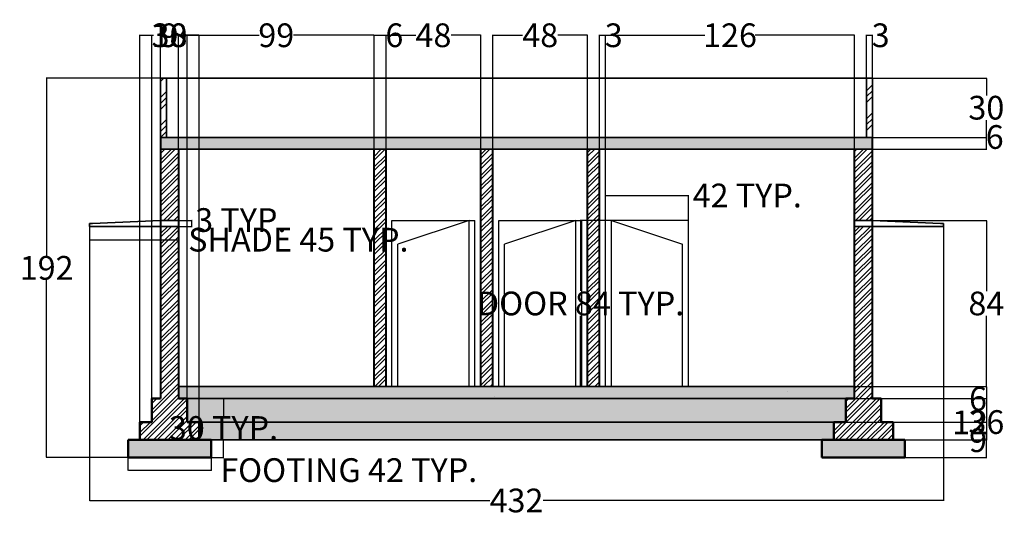
# Model space of a CAD drawing. Units: inches. Extents: x -51 to 1196, y -40 to 252.
# Tile 1 of 2: x -51 to 447, y -40 to 215. Entities that reach past the tile are written whole.
import ezdxf

# ---------------------------------------------------------------- set-up
doc = ezdxf.new("R2010")
doc.units = ezdxf.units.IN
doc.header["$MEASUREMENT"] = 0
for name, color, linetype, lineweight in [('A-ANNO-DIMS', 2, 'Continuous', 18), ('A-DOOR', 4, 'Continuous', 25), ('A-FLOR', 7, 'Continuous', 35), ('A-FLOR-PATT', 8, 'Continuous', 13), ('A-ROOF', 7, 'Continuous', 35), ('A-ROOF-PATT', 8, 'Continuous', 13), ('A-SECT-PATT', 8, 'Continuous', 13), ('A-WALL', 7, 'Continuous', 40), ('S-FNDN', 1, 'Continuous', 50), ('S-FNDN-PATT', 8, 'Continuous', 13)]:
    doc.layers.add(name, color=color, linetype=linetype, lineweight=lineweight)
doc.styles.get("Standard").update_dxf_attribs({"font": 'arial.ttf'})
doc.dimstyles.get("Standard").update_dxf_attribs({"dimtxt": 12, "dimasz": 0.18, "dimexe": 0.18, "dimexo": 0.0625, "dimgap": 0.09, "dimtad": 0, "dimtih": 1, "dimtoh": 1, "dimdec": 0, "dimzin": 0, "dimdsep": 46, "dimlunit": 4, "dimtxsty": 'Standard', "dimcen": 0.09, "dimadec": 0, "dimazin": 0, "dimtfac": 1, "dimtdec": 0, "dimtofl": 0, "dimtmove": 0, "dimatfit": 3, "dimfxl": 1, "dimtolj": 1, "dimtzin": 0, "dimarcsym": 0})

# ---------------------------------------------------------------- blocks, each defined once
blk = doc.blocks.new('DOOR-42X84-SECTION')
for p, q in [((42, 84), (0, 84)), ((0, 0), (0, 84)), ((3, 0), (3, 84)), ((3, 84), (39, 72)), ((42, 0), (42, 84)), ((39, 0), (39, 72))]:
    blk.add_line(p, q)
blk = doc.blocks.new('FOOTING-STEPPED-42')
for p, q in [((12, 30), (12, 18)), ((16.5, 30), (12, 30)), ((30, 30), (25.5, 30)), ((30, 18), (30, 30)), ((12, 18), (6, 18)), ((6, 18), (6, 9)), ((36, 18), (30, 18)), ((36, 9), (36, 18)), ((6, 9), (0, 9)), ((0, 9), (0, 0)), ((6, 9), (36, 9)), ((42, 9), (36, 9)), ((42, 0), (42, 9)), ((0, 0), (42, 0))]:
    blk.add_line(p, q)
blk = doc.blocks.new('SHADE-PROJECTING-36')
for p, q in [((0, 0), (0, 1.5)), ((0, 1.5), (1.5, 1.5)), ((36, 0), (0, 0)), ((1.5, 1.5), (36, 3)), ((45, 3), (36, 3)), ((45, 0), (36, 0))]:
    blk.add_line(p, q)
blk = doc.blocks.new('*D6')
at = {"layer": 'A-ANNO-DIMS', "color": 0, "lineweight": -2, "transparency": 16777216}
for p, q in [((245.36, 113.83), (232.64, 113.83)), ((232.82, 113.65), (232.82, 78.13)), ((232.82, 30.01), (232.82, 65.53)), ((245.36, 29.83), (232.64, 29.83))]:
    blk.add_line(p, q, dxfattribs=at)
at = {"layer": 'A-ANNO-DIMS', "color": 0, "transparency": 16777216}
for points in [[(232.79, 113.65), (232.85, 113.65), (232.82, 113.83)], [(232.79, 30.01), (232.85, 30.01), (232.82, 29.83)]]:
    blk.add_solid(points, dxfattribs=at)
at = {"layer": 'Defpoints', "color": 0, "transparency": 16777216}
for p in [(232.82, 113.83), (245.42, 113.83), (245.42, 29.83)]:
    blk.add_point(p, dxfattribs=at)
at = {"layer": 'A-ANNO-DIMS', "color": 0, "transparency": 16777216, "insert": (232.82, 71.83), "char_height": 12, "attachment_point": 5}
blk.add_mtext('\\A1;DOOR 84 TYP.', dxfattribs=at)
blk = doc.blocks.new('*D7')
at = {"layer": 'A-ANNO-DIMS', "color": 0, "lineweight": -2, "transparency": 16777216}
for p, q in [((245.42, 113.89), (245.42, 126.61)), ((245.6, 126.43), (287.24, 126.43)), ((287.42, 113.89), (287.42, 126.61)), ((287.42, 126.43), (287.6, 126.43))]:
    blk.add_line(p, q, dxfattribs=at)
at = {"layer": 'A-ANNO-DIMS', "color": 0, "transparency": 16777216}
for points in [[(245.6, 126.46), (245.6, 126.4), (245.42, 126.43)], [(287.24, 126.46), (287.24, 126.4), (287.42, 126.43)]]:
    blk.add_solid(points, dxfattribs=at)
at = {"layer": 'Defpoints', "color": 0, "transparency": 16777216}
for p in [(287.42, 126.43), (245.42, 113.83), (287.42, 113.83)]:
    blk.add_point(p, dxfattribs=at)
at = {"layer": 'A-ANNO-DIMS', "color": 0, "transparency": 16777216, "insert": (317.14, 126.43), "char_height": 12, "attachment_point": 5}
blk.add_mtext('\\A1;42 TYP.', dxfattribs=at)
blk = doc.blocks.new('*D8')
at = {"layer": 'A-ANNO-DIMS', "color": 0, "lineweight": -2, "transparency": 16777216}
for p, q in [((3.92, -6.24), (3.92, -12.65)), ((45.92, -6.24), (45.92, -12.65)), ((4.1, -12.47), (45.74, -12.47)), ((45.92, -12.47), (46.1, -12.47))]:
    blk.add_line(p, q, dxfattribs=at)
at = {"layer": 'A-ANNO-DIMS', "color": 0, "transparency": 16777216}
for points in [[(4.1, -12.44), (4.1, -12.5), (3.92, -12.47)], [(45.74, -12.44), (45.74, -12.5), (45.92, -12.47)]]:
    blk.add_solid(points, dxfattribs=at)
at = {"layer": 'Defpoints', "color": 0, "transparency": 16777216}
for p in [(3.92, -6.17), (45.92, -6.17), (45.92, -12.47)]:
    blk.add_point(p, dxfattribs=at)
at = {"layer": 'A-ANNO-DIMS', "color": 0, "transparency": 16777216, "insert": (115.57, -12.47), "char_height": 12, "attachment_point": 5}
blk.add_mtext('\\A1;FOOTING 42 TYP.', dxfattribs=at)
blk = doc.blocks.new('*D9')
at = {"layer": 'A-ANNO-DIMS', "color": 0, "lineweight": -2, "transparency": 16777216}
for p, q in [((45.98, 23.83), (52.4, 23.83)), ((52.22, 23.65), (52.22, 15.05)), ((52.22, -5.99), (52.22, 2.61)), ((45.98, -6.17), (52.4, -6.17))]:
    blk.add_line(p, q, dxfattribs=at)
at = {"layer": 'A-ANNO-DIMS', "color": 0, "transparency": 16777216}
for points in [[(52.19, 23.65), (52.25, 23.65), (52.22, 23.83)], [(52.19, -5.99), (52.25, -5.99), (52.22, -6.17)]]:
    blk.add_solid(points, dxfattribs=at)
at = {"layer": 'Defpoints', "color": 0, "transparency": 16777216}
for p in [(45.92, 23.83), (52.22, 23.83), (45.92, -6.17)]:
    blk.add_point(p, dxfattribs=at)
at = {"layer": 'A-ANNO-DIMS', "color": 0, "transparency": 16777216, "insert": (52.22, 8.83), "char_height": 12, "attachment_point": 5}
blk.add_mtext('\\A1;30 TYP.', dxfattribs=at)
blk = doc.blocks.new('*D10')
at = {"layer": 'A-ANNO-DIMS', "color": 0, "lineweight": -2, "transparency": 16777216}
for p, q in [((-15.58, 110.76), (-15.58, 103.9)), ((29.42, 110.76), (29.42, 103.9)), ((-15.4, 104.08), (29.24, 104.08)), ((29.42, 104.08), (29.6, 104.08))]:
    blk.add_line(p, q, dxfattribs=at)
at = {"layer": 'A-ANNO-DIMS', "color": 0, "transparency": 16777216}
for points in [[(-15.4, 104.11), (-15.4, 104.05), (-15.58, 104.08)], [(29.24, 104.11), (29.24, 104.05), (29.42, 104.08)]]:
    blk.add_solid(points, dxfattribs=at)
at = {"layer": 'Defpoints', "color": 0, "transparency": 16777216}
for p in [(-15.58, 110.83), (29.42, 110.83), (29.42, 104.08)]:
    blk.add_point(p, dxfattribs=at)
at = {"layer": 'A-ANNO-DIMS', "color": 0, "transparency": 16777216, "insert": (90.08, 104.08), "char_height": 12, "attachment_point": 5}
blk.add_mtext('\\A1;SHADE 45 TYP.', dxfattribs=at)
blk = doc.blocks.new('*D11')
at = {"layer": 'A-ANNO-DIMS', "color": 0, "lineweight": -2, "transparency": 16777216}
for p, q in [((29.48, 113.83), (36.35, 113.83)), ((29.48, 110.83), (36.35, 110.83)), ((36.17, 113.83), (36.17, 114.01)), ((36.17, 114.01), (36.35, 114.01)), ((36.17, 111.01), (36.17, 113.65))]:
    blk.add_line(p, q, dxfattribs=at)
at = {"layer": 'A-ANNO-DIMS', "color": 0, "transparency": 16777216}
for points in [[(36.14, 113.65), (36.2, 113.65), (36.17, 113.83)], [(36.14, 111.01), (36.2, 111.01), (36.17, 110.83)]]:
    blk.add_solid(points, dxfattribs=at)
at = {"layer": 'Defpoints', "color": 0, "transparency": 16777216}
for p in [(29.42, 113.83), (29.42, 110.83), (36.17, 113.83)]:
    blk.add_point(p, dxfattribs=at)
at = {"layer": 'A-ANNO-DIMS', "color": 0, "transparency": 16777216, "insert": (60.98, 114.01), "char_height": 12, "attachment_point": 5}
blk.add_mtext('\\A1;3 TYP.', dxfattribs=at)
blk = doc.blocks.new('*D16')
at = {"layer": 'A-ANNO-DIMS', "color": 0, "lineweight": -2, "transparency": 16777216}
for p, q in [((-15.58, 110.76), (-15.58, -28.01)), ((416.42, 110.76), (416.42, -28.01)), ((-15.4, -27.83), (186.9, -27.83)), ((416.24, -27.83), (213.95, -27.83))]:
    blk.add_line(p, q, dxfattribs=at)
at = {"layer": 'A-ANNO-DIMS', "color": 0, "transparency": 16777216}
for points in [[(-15.4, -27.8), (-15.4, -27.86), (-15.58, -27.83)], [(416.24, -27.8), (416.24, -27.86), (416.42, -27.83)]]:
    blk.add_solid(points, dxfattribs=at)
at = {"layer": 'Defpoints', "color": 0, "transparency": 16777216}
for p in [(-15.58, 110.83), (416.42, 110.83), (416.42, -27.83)]:
    blk.add_point(p, dxfattribs=at)
at = {"layer": 'A-ANNO-DIMS', "color": 0, "transparency": 16777216, "insert": (200.42, -27.83), "char_height": 12, "attachment_point": 5}
blk.add_mtext('\\A1;432', dxfattribs=at)
blk = doc.blocks.new('*D17')
at = {"layer": 'A-ANNO-DIMS', "color": 0, "lineweight": -2, "transparency": 16777216}
for p, q in [((20.36, 185.83), (-37.41, 185.83)), ((-37.23, 185.65), (-37.23, 96.04)), ((-37.23, -5.99), (-37.23, 83.61)), ((3.86, -6.17), (-37.41, -6.17))]:
    blk.add_line(p, q, dxfattribs=at)
at = {"layer": 'A-ANNO-DIMS', "color": 0, "transparency": 16777216}
for points in [[(-37.26, 185.65), (-37.2, 185.65), (-37.23, 185.83)], [(-37.26, -5.99), (-37.2, -5.99), (-37.23, -6.17)]]:
    blk.add_solid(points, dxfattribs=at)
at = {"layer": 'Defpoints', "color": 0, "transparency": 16777216}
for p in [(20.42, 185.83), (-37.23, -6.17), (3.92, -6.17)]:
    blk.add_point(p, dxfattribs=at)
at = {"layer": 'A-ANNO-DIMS', "color": 0, "transparency": 16777216, "insert": (-37.23, 89.83), "char_height": 12, "attachment_point": 5}
blk.add_mtext('\\A1;192', dxfattribs=at)
blk = doc.blocks.new('*D18')
at = {"layer": 'A-ANNO-DIMS', "color": 0, "lineweight": -2, "transparency": 16777216}
for p, q in [((371.48, 29.83), (438.26, 29.83)), ((438.08, 29.65), (438.08, 18.05)), ((438.08, -5.99), (438.08, 5.61)), ((396.98, -6.17), (438.26, -6.17))]:
    blk.add_line(p, q, dxfattribs=at)
at = {"layer": 'A-ANNO-DIMS', "color": 0, "transparency": 16777216}
for points in [[(438.05, 29.65), (438.11, 29.65), (438.08, 29.83)], [(438.05, -5.99), (438.11, -5.99), (438.08, -6.17)]]:
    blk.add_solid(points, dxfattribs=at)
at = {"layer": 'Defpoints', "color": 0, "transparency": 16777216}
for p in [(371.42, 29.83), (438.08, 29.83), (396.92, -6.17)]:
    blk.add_point(p, dxfattribs=at)
at = {"layer": 'A-ANNO-DIMS', "color": 0, "transparency": 16777216, "insert": (438.08, 11.83), "char_height": 12, "attachment_point": 5}
blk.add_mtext('\\A1;36', dxfattribs=at)
blk = doc.blocks.new('*D19')
at = {"layer": 'A-ANNO-DIMS', "color": 0, "lineweight": -2, "transparency": 16777216}
for p, q in [((380.48, 113.83), (438.26, 113.83)), ((438.08, 113.65), (438.08, 78.04)), ((438.08, 30.01), (438.08, 65.61)), ((371.48, 29.83), (438.26, 29.83))]:
    blk.add_line(p, q, dxfattribs=at)
at = {"layer": 'A-ANNO-DIMS', "color": 0, "transparency": 16777216}
for points in [[(438.05, 113.65), (438.11, 113.65), (438.08, 113.83)], [(438.05, 30.01), (438.11, 30.01), (438.08, 29.83)]]:
    blk.add_solid(points, dxfattribs=at)
at = {"layer": 'Defpoints', "color": 0, "transparency": 16777216}
for p in [(380.42, 113.83), (438.08, 113.83), (371.42, 29.83)]:
    blk.add_point(p, dxfattribs=at)
at = {"layer": 'A-ANNO-DIMS', "color": 0, "transparency": 16777216, "insert": (438.08, 71.83), "char_height": 12, "attachment_point": 5}
blk.add_mtext('\\A1;84', dxfattribs=at)
blk = doc.blocks.new('*D20')
at = {"layer": 'A-ANNO-DIMS', "color": 0, "lineweight": -2, "transparency": 16777216}
for p, q in [((380.48, 155.83), (438.26, 155.83)), ((438.08, 155.83), (438.08, 156.01)), ((438.08, 156.01), (438.26, 156.01)), ((438.08, 150.01), (438.08, 155.65)), ((380.48, 149.83), (438.26, 149.83))]:
    blk.add_line(p, q, dxfattribs=at)
at = {"layer": 'A-ANNO-DIMS', "color": 0, "transparency": 16777216}
for points in [[(438.05, 155.65), (438.11, 155.65), (438.08, 155.83)], [(438.05, 150.01), (438.11, 150.01), (438.08, 149.83)]]:
    blk.add_solid(points, dxfattribs=at)
at = {"layer": 'Defpoints', "color": 0, "transparency": 16777216}
for p in [(380.42, 155.83), (438.08, 155.83), (380.42, 149.83)]:
    blk.add_point(p, dxfattribs=at)
at = {"layer": 'A-ANNO-DIMS', "color": 0, "transparency": 16777216, "insert": (442.31, 156.01), "char_height": 12, "attachment_point": 5}
blk.add_mtext('\\A1;6', dxfattribs=at)
blk = doc.blocks.new('*D21')
at = {"layer": 'A-ANNO-DIMS', "color": 0, "lineweight": -2, "transparency": 16777216}
for p, q in [((380.48, 185.83), (438.26, 185.83)), ((438.08, 185.65), (438.08, 177.05)), ((438.08, 156.01), (438.08, 164.61)), ((380.48, 155.83), (438.26, 155.83))]:
    blk.add_line(p, q, dxfattribs=at)
at = {"layer": 'A-ANNO-DIMS', "color": 0, "transparency": 16777216}
for points in [[(438.05, 185.65), (438.11, 185.65), (438.08, 185.83)], [(438.05, 156.01), (438.11, 156.01), (438.08, 155.83)]]:
    blk.add_solid(points, dxfattribs=at)
at = {"layer": 'Defpoints', "color": 0, "transparency": 16777216}
for p in [(380.42, 185.83), (438.08, 185.83), (380.42, 155.83)]:
    blk.add_point(p, dxfattribs=at)
at = {"layer": 'A-ANNO-DIMS', "color": 0, "transparency": 16777216, "insert": (438.08, 170.83), "char_height": 12, "attachment_point": 5}
blk.add_mtext('\\A1;30', dxfattribs=at)
blk = doc.blocks.new('*D22')
at = {"layer": 'A-ANNO-DIMS', "color": 0, "lineweight": -2, "transparency": 16777216}
for p, q in [((20.42, 149.89), (20.42, 207.66)), ((20.6, 207.48), (20.89, 207.48)), ((29.24, 207.48), (28.96, 207.48)), ((29.42, 149.89), (29.42, 207.66))]:
    blk.add_line(p, q, dxfattribs=at)
at = {"layer": 'A-ANNO-DIMS', "color": 0, "transparency": 16777216}
for points in [[(20.6, 207.51), (20.6, 207.45), (20.42, 207.48)], [(29.24, 207.51), (29.24, 207.45), (29.42, 207.48)]]:
    blk.add_solid(points, dxfattribs=at)
at = {"layer": 'Defpoints', "color": 0, "transparency": 16777216}
for p in [(29.42, 207.48), (20.42, 149.83), (29.42, 149.83)]:
    blk.add_point(p, dxfattribs=at)
at = {"layer": 'A-ANNO-DIMS', "color": 0, "transparency": 16777216, "insert": (24.92, 207.48), "char_height": 12, "attachment_point": 5}
blk.add_mtext('\\A1;9', dxfattribs=at)
blk = doc.blocks.new('*D23')
at = {"layer": 'A-ANNO-DIMS', "color": 0, "lineweight": -2, "transparency": 16777216}
for p, q in [((29.42, 149.89), (29.42, 207.66)), ((29.6, 207.48), (70.22, 207.48)), ((128.24, 207.48), (87.62, 207.48)), ((128.42, 149.89), (128.42, 207.66))]:
    blk.add_line(p, q, dxfattribs=at)
at = {"layer": 'A-ANNO-DIMS', "color": 0, "transparency": 16777216}
for points in [[(29.6, 207.51), (29.6, 207.45), (29.42, 207.48)], [(128.24, 207.51), (128.24, 207.45), (128.42, 207.48)]]:
    blk.add_solid(points, dxfattribs=at)
at = {"layer": 'Defpoints', "color": 0, "transparency": 16777216}
for p in [(128.42, 207.48), (29.42, 149.83), (128.42, 149.83)]:
    blk.add_point(p, dxfattribs=at)
at = {"layer": 'A-ANNO-DIMS', "color": 0, "transparency": 16777216, "insert": (78.92, 207.48), "char_height": 12, "attachment_point": 5}
blk.add_mtext('\\A1;99', dxfattribs=at)
blk = doc.blocks.new('*D24')
at = {"layer": 'A-ANNO-DIMS', "color": 0, "lineweight": -2, "transparency": 16777216}
for p, q in [((128.42, 149.89), (128.42, 207.66)), ((128.6, 207.48), (134.24, 207.48)), ((134.42, 149.89), (134.42, 207.66)), ((134.42, 207.48), (134.6, 207.48))]:
    blk.add_line(p, q, dxfattribs=at)
at = {"layer": 'A-ANNO-DIMS', "color": 0, "transparency": 16777216}
for points in [[(128.6, 207.51), (128.6, 207.45), (128.42, 207.48)], [(134.24, 207.51), (134.24, 207.45), (134.42, 207.48)]]:
    blk.add_solid(points, dxfattribs=at)
at = {"layer": 'Defpoints', "color": 0, "transparency": 16777216}
for p in [(134.42, 207.48), (128.42, 149.83), (134.42, 149.83)]:
    blk.add_point(p, dxfattribs=at)
at = {"layer": 'A-ANNO-DIMS', "color": 0, "transparency": 16777216, "insert": (138.65, 207.48), "char_height": 12, "attachment_point": 5}
blk.add_mtext('\\A1;6', dxfattribs=at)
blk = doc.blocks.new('*D25')
at = {"layer": 'A-ANNO-DIMS', "color": 0, "lineweight": -2, "transparency": 16777216}
for p, q in [((134.42, 149.89), (134.42, 207.66)), ((134.6, 207.48), (149.48, 207.48)), ((182.24, 207.48), (167.36, 207.48)), ((182.42, 149.89), (182.42, 207.66))]:
    blk.add_line(p, q, dxfattribs=at)
at = {"layer": 'A-ANNO-DIMS', "color": 0, "transparency": 16777216}
for points in [[(134.6, 207.51), (134.6, 207.45), (134.42, 207.48)], [(182.24, 207.51), (182.24, 207.45), (182.42, 207.48)]]:
    blk.add_solid(points, dxfattribs=at)
at = {"layer": 'Defpoints', "color": 0, "transparency": 16777216}
for p in [(182.42, 207.48), (134.42, 149.83), (182.42, 149.83)]:
    blk.add_point(p, dxfattribs=at)
at = {"layer": 'A-ANNO-DIMS', "color": 0, "transparency": 16777216, "insert": (158.42, 207.48), "char_height": 12, "attachment_point": 5}
blk.add_mtext('\\A1;48', dxfattribs=at)
blk = doc.blocks.new('*D26')
at = {"layer": 'A-ANNO-DIMS', "color": 0, "lineweight": -2, "transparency": 16777216}
for p, q in [((188.42, 149.89), (188.42, 207.66)), ((188.6, 207.48), (203.48, 207.48)), ((236.24, 207.48), (221.36, 207.48)), ((236.42, 149.89), (236.42, 207.66))]:
    blk.add_line(p, q, dxfattribs=at)
at = {"layer": 'A-ANNO-DIMS', "color": 0, "transparency": 16777216}
for points in [[(188.6, 207.51), (188.6, 207.45), (188.42, 207.48)], [(236.24, 207.51), (236.24, 207.45), (236.42, 207.48)]]:
    blk.add_solid(points, dxfattribs=at)
at = {"layer": 'Defpoints', "color": 0, "transparency": 16777216}
for p in [(236.42, 207.48), (188.42, 149.83), (236.42, 149.83)]:
    blk.add_point(p, dxfattribs=at)
at = {"layer": 'A-ANNO-DIMS', "color": 0, "transparency": 16777216, "insert": (212.42, 207.48), "char_height": 12, "attachment_point": 5}
blk.add_mtext('\\A1;48', dxfattribs=at)
blk = doc.blocks.new('*D27')
at = {"layer": 'A-ANNO-DIMS', "color": 0, "lineweight": -2, "transparency": 16777216}
for p, q in [((242.42, 149.89), (242.42, 207.66)), ((242.6, 207.48), (245.24, 207.48)), ((245.42, 113.89), (245.42, 207.66)), ((245.42, 207.48), (245.6, 207.48))]:
    blk.add_line(p, q, dxfattribs=at)
at = {"layer": 'A-ANNO-DIMS', "color": 0, "transparency": 16777216}
for points in [[(242.6, 207.51), (242.6, 207.45), (242.42, 207.48)], [(245.24, 207.51), (245.24, 207.45), (245.42, 207.48)]]:
    blk.add_solid(points, dxfattribs=at)
at = {"layer": 'Defpoints', "color": 0, "transparency": 16777216}
for p in [(245.42, 207.48), (242.42, 149.83), (245.42, 113.83)]:
    blk.add_point(p, dxfattribs=at)
at = {"layer": 'A-ANNO-DIMS', "color": 0, "transparency": 16777216, "insert": (249.62, 207.48), "char_height": 12, "attachment_point": 5}
blk.add_mtext('\\A1;3', dxfattribs=at)
blk = doc.blocks.new('*D28')
at = {"layer": 'A-ANNO-DIMS', "color": 0, "lineweight": -2, "transparency": 16777216}
for p, q in [((245.42, 113.89), (245.42, 207.66)), ((245.6, 207.48), (295.64, 207.48)), ((371.24, 207.48), (321.2, 207.48)), ((371.42, 149.89), (371.42, 207.66))]:
    blk.add_line(p, q, dxfattribs=at)
at = {"layer": 'A-ANNO-DIMS', "color": 0, "transparency": 16777216}
for points in [[(245.6, 207.51), (245.6, 207.45), (245.42, 207.48)], [(371.24, 207.51), (371.24, 207.45), (371.42, 207.48)]]:
    blk.add_solid(points, dxfattribs=at)
at = {"layer": 'Defpoints', "color": 0, "transparency": 16777216}
for p in [(371.42, 207.48), (371.42, 149.83), (245.42, 113.83)]:
    blk.add_point(p, dxfattribs=at)
at = {"layer": 'A-ANNO-DIMS', "color": 0, "transparency": 16777216, "insert": (308.42, 207.48), "char_height": 12, "attachment_point": 5}
blk.add_mtext('\\A1;126', dxfattribs=at)
blk = doc.blocks.new('*D29')
at = {"layer": 'A-ANNO-DIMS', "color": 0, "lineweight": -2, "transparency": 16777216}
for p, q in [((377.42, 185.89), (377.42, 207.66)), ((377.6, 207.48), (380.24, 207.48)), ((380.42, 185.89), (380.42, 207.66)), ((380.42, 207.48), (380.6, 207.48))]:
    blk.add_line(p, q, dxfattribs=at)
at = {"layer": 'A-ANNO-DIMS', "color": 0, "transparency": 16777216}
for points in [[(377.6, 207.51), (377.6, 207.45), (377.42, 207.48)], [(380.24, 207.51), (380.24, 207.45), (380.42, 207.48)]]:
    blk.add_solid(points, dxfattribs=at)
at = {"layer": 'Defpoints', "color": 0, "transparency": 16777216}
for p in [(380.42, 207.48), (377.42, 185.83), (380.42, 185.83)]:
    blk.add_point(p, dxfattribs=at)
at = {"layer": 'A-ANNO-DIMS', "color": 0, "transparency": 16777216, "insert": (384.62, 207.48), "char_height": 12, "attachment_point": 5}
blk.add_mtext('\\A1;3', dxfattribs=at)
blk = doc.blocks.new('*D30')
at = {"layer": 'A-ANNO-DIMS', "color": 0, "lineweight": -2, "transparency": 16777216}
for p, q in [((29.48, 29.83), (438.26, 29.83)), ((438.08, 29.65), (438.08, 24.01)), ((33.98, 23.83), (438.26, 23.83)), ((438.08, 23.65), (437.9, 23.65)), ((438.08, 23.83), (438.08, 23.65))]:
    blk.add_line(p, q, dxfattribs=at)
at = {"layer": 'A-ANNO-DIMS', "color": 0, "transparency": 16777216}
for points in [[(438.05, 29.65), (438.11, 29.65), (438.08, 29.83)], [(438.05, 24.01), (438.11, 24.01), (438.08, 23.83)]]:
    blk.add_solid(points, dxfattribs=at)
at = {"layer": 'Defpoints', "color": 0, "transparency": 16777216}
for p in [(29.42, 29.83), (33.92, 23.83), (438.08, 23.83)]:
    blk.add_point(p, dxfattribs=at)
at = {"layer": 'A-ANNO-DIMS', "color": 0, "transparency": 16777216, "insert": (433.85, 23.65), "char_height": 12, "attachment_point": 5}
blk.add_mtext('\\A1;6', dxfattribs=at)
blk = doc.blocks.new('*D31')
at = {"layer": 'A-ANNO-DIMS', "color": 0, "lineweight": -2, "transparency": 16777216}
for p, q in [((33.98, 23.83), (438.26, 23.83)), ((438.08, 23.65), (438.08, 12.01)), ((33.98, 11.83), (438.26, 11.83)), ((438.08, 11.65), (437.9, 11.65)), ((438.08, 11.83), (438.08, 11.65))]:
    blk.add_line(p, q, dxfattribs=at)
at = {"layer": 'A-ANNO-DIMS', "color": 0, "transparency": 16777216}
for points in [[(438.05, 23.65), (438.11, 23.65), (438.08, 23.83)], [(438.05, 12.01), (438.11, 12.01), (438.08, 11.83)]]:
    blk.add_solid(points, dxfattribs=at)
at = {"layer": 'Defpoints', "color": 0, "transparency": 16777216}
for p in [(33.92, 23.83), (33.92, 11.83), (438.08, 11.83)]:
    blk.add_point(p, dxfattribs=at)
at = {"layer": 'A-ANNO-DIMS', "color": 0, "transparency": 16777216, "insert": (429.84, 11.65), "char_height": 12, "attachment_point": 5}
blk.add_mtext('\\A1;12', dxfattribs=at)
blk = doc.blocks.new('*D32')
at = {"layer": 'A-ANNO-DIMS', "color": 0, "lineweight": -2, "transparency": 16777216}
for p, q in [((39.98, 11.83), (438.26, 11.83)), ((438.08, 11.65), (438.08, 3.01)), ((39.98, 2.83), (438.26, 2.83)), ((438.08, 2.65), (437.9, 2.65)), ((438.08, 2.83), (438.08, 2.65))]:
    blk.add_line(p, q, dxfattribs=at)
at = {"layer": 'A-ANNO-DIMS', "color": 0, "transparency": 16777216}
for points in [[(438.05, 11.65), (438.11, 11.65), (438.08, 11.83)], [(438.05, 3.01), (438.11, 3.01), (438.08, 2.83)]]:
    blk.add_solid(points, dxfattribs=at)
at = {"layer": 'Defpoints', "color": 0, "transparency": 16777216}
for p in [(39.92, 11.83), (39.92, 2.83), (438.08, 2.83)]:
    blk.add_point(p, dxfattribs=at)
at = {"layer": 'A-ANNO-DIMS', "color": 0, "transparency": 16777216, "insert": (433.86, 2.65), "char_height": 12, "attachment_point": 5}
blk.add_mtext('\\A1;9', dxfattribs=at)
blk = doc.blocks.new('*D33')
at = {"layer": 'A-ANNO-DIMS', "color": 0, "lineweight": -2, "transparency": 16777216}
for p, q in [((9.92, 2.89), (9.92, 207.66)), ((10.1, 207.48), (16.26, 207.48)), ((39.74, 207.48), (33.58, 207.48)), ((39.92, 2.89), (39.92, 207.66))]:
    blk.add_line(p, q, dxfattribs=at)
at = {"layer": 'A-ANNO-DIMS', "color": 0, "transparency": 16777216}
for points in [[(10.1, 207.51), (10.1, 207.45), (9.92, 207.48)], [(39.74, 207.51), (39.74, 207.45), (39.92, 207.48)]]:
    blk.add_solid(points, dxfattribs=at)
at = {"layer": 'Defpoints', "color": 0, "transparency": 16777216}
for p in [(39.92, 207.48), (9.92, 2.83), (39.92, 2.83)]:
    blk.add_point(p, dxfattribs=at)
at = {"layer": 'A-ANNO-DIMS', "color": 0, "transparency": 16777216, "insert": (24.92, 207.48), "char_height": 12, "attachment_point": 5}
blk.add_mtext('\\A1;30', dxfattribs=at)
blk = doc.blocks.new('*D34')
at = {"layer": 'A-ANNO-DIMS', "color": 0, "lineweight": -2, "transparency": 16777216}
for p, q in [((15.92, 23.89), (15.92, 207.66)), ((16.1, 207.48), (16.79, 207.48)), ((33.74, 207.48), (33.05, 207.48)), ((33.92, 23.89), (33.92, 207.66))]:
    blk.add_line(p, q, dxfattribs=at)
at = {"layer": 'A-ANNO-DIMS', "color": 0, "transparency": 16777216}
for points in [[(16.1, 207.51), (16.1, 207.45), (15.92, 207.48)], [(33.74, 207.51), (33.74, 207.45), (33.92, 207.48)]]:
    blk.add_solid(points, dxfattribs=at)
at = {"layer": 'Defpoints', "color": 0, "transparency": 16777216}
for p in [(33.92, 207.48), (15.92, 23.83), (33.92, 23.83)]:
    blk.add_point(p, dxfattribs=at)
at = {"layer": 'A-ANNO-DIMS', "color": 0, "transparency": 16777216, "insert": (24.92, 207.48), "char_height": 12, "attachment_point": 5}
blk.add_mtext('\\A1;18', dxfattribs=at)

msp = doc.modelspace()

# ---------------------------------------------------------------- hatches: boundary and pattern name
at = {"layer": 'A-FLOR-PATT'}
h = msp.add_hatch(dxfattribs=at)
h.set_pattern_fill('AR-CONC', color=256, scale=15)
h.paths.add_polyline_path([(371.422, 29.8273), (29.422, 29.8273), (29.422, 23.8273), (33.922, 23.8273), (371.422, 23.8273)])
h = msp.add_hatch(dxfattribs=at)
h.set_pattern_fill('AR-CONC', color=256, scale=15)
h.paths.add_polyline_path([(371.422, 29.8273), (29.422, 29.8273), (29.422, 23.8273), (33.922, 23.8273), (371.422, 23.8273)])
h = msp.add_hatch(dxfattribs=at)
h.set_pattern_fill('AR-SAND', color=256, scale=2)
h.paths.add_polyline_path([(366.922, 23.8273), (33.922, 23.8273), (33.922, 11.8273), (39.922, 11.8273), (360.922, 11.8273), (366.922, 11.8273)])
h = msp.add_hatch(dxfattribs=at)
h.set_pattern_fill('HONEY', color=256, scale=20)
h.paths.add_polyline_path([(360.922, 11.8273), (39.922, 11.8273), (39.922, 2.8273), (45.922, 2.8273), (354.922, 2.8273), (360.922, 2.8273)])
at = {"layer": 'A-ROOF-PATT'}
h = msp.add_hatch(dxfattribs=at)
h.set_pattern_fill('GOST_GROUND', color=256)
h.set_pattern_definition([(45, (0, 0), (14.14214, 0), [20]), (45, (3, 0), (14.14214, 0), [20]), (45, (6, 0), (14.14214, 0), [20])])
h.paths.add_polyline_path([(23.422, 185.8273), (20.422, 185.8273), (20.422, 155.8273), (23.422, 155.8273)])
h.paths.add_polyline_path([(380.422, 185.8273), (377.422, 185.8273), (377.422, 155.8273), (380.422, 155.8273)])
at = {"layer": 'A-SECT-PATT'}
h = msp.add_hatch(dxfattribs=at)
h.set_pattern_fill('AR-CONC', color=256, scale=2)
h.paths.add_polyline_path([(371.422, 29.8273), (29.422, 29.8273), (29.422, 23.8273), (33.922, 23.8273), (371.422, 23.8273)])
h.paths.add_polyline_path([(366.922, 23.8273), (33.922, 23.8273), (33.922, 11.8273), (39.922, 11.8273), (360.922, 11.8273), (366.922, 11.8273)])
h.paths.add_polyline_path([(380.422, 155.8273), (377.422, 155.8273), (20.422, 155.8273), (20.422, 149.8273), (380.422, 149.8273)])
h = msp.add_hatch(dxfattribs=at)
h.set_pattern_fill('STEEL', color=256, scale=30)
h.set_pattern_definition([(45, (0, 0), (-2.65165, 2.65165), []), (45, (0, 1.875), (-2.65165, 2.65165), [])])
h.paths.add_polyline_path([(29.422, 110.8273), (20.422, 110.8273), (20.422, 23.8273), (15.922, 23.8273), (15.922, 11.8273), (9.922, 11.8273), (9.922, 2.8273), (39.922, 2.8273), (39.922, 11.8273), (33.922, 11.8273), (33.922, 23.8273), (29.422, 23.8273)])
h.paths.add_polyline_path([(29.422, 149.8273), (20.422, 149.8273), (20.422, 113.8273), (29.422, 113.8273)])
h.paths.add_polyline_path([(134.422, 149.8273), (128.422, 149.8273), (128.422, 29.8273), (134.422, 29.8273)])
h.paths.add_polyline_path([(188.422, 149.8273), (182.422, 149.8273), (182.422, 29.8273), (188.422, 29.8273)])
h.paths.add_polyline_path([(242.422, 149.8273), (236.422, 149.8273), (236.422, 29.8273), (242.422, 29.8273)])
h.paths.add_polyline_path([(380.422, 110.8273), (371.422, 110.8273), (371.422, 29.8273), (371.422, 23.8273), (366.922, 23.8273), (366.922, 11.8273), (360.922, 11.8273), (360.922, 2.8273), (390.922, 2.8273), (390.922, 11.8273), (384.922, 11.8273), (384.922, 23.8273), (380.422, 23.8273), (380.422, 29.8273)])
h.paths.add_polyline_path([(380.422, 149.8273), (371.422, 149.8273), (371.422, 113.8273), (380.422, 113.8273)])
at = {"layer": 'S-FNDN-PATT'}
h = msp.add_hatch(dxfattribs=at)
h.set_pattern_fill('AR-SAND', color=256, scale=2)
h.paths.add_polyline_path([(45.922, 2.8273), (39.922, 2.8273), (9.922, 2.8273), (3.922, 2.8273), (3.922, -6.1727), (45.922, -6.1727)])
h.paths.add_polyline_path([(396.922, 2.8273), (390.922, 2.8273), (360.922, 2.8273), (354.922, 2.8273), (354.922, -6.1727), (396.922, -6.1727)])

# ---------------------------------------------------------------- linework, layer by layer
at = {"layer": 'A-FLOR'}
for p, q in [((371.422, 29.8273), (29.422, 29.8273)), ((371.422, 23.8273), (29.422, 23.8273)), ((39.922, 11.8273), (360.922, 11.8273)), ((354.922, 2.8273), (45.922, 2.8273))]:
    msp.add_line(p, q, dxfattribs=at)
at = {"layer": 'A-ROOF'}
for p, q in [((23.422, 185.8273), (377.422, 185.8273)), ((380.422, 155.8273), (20.422, 155.8273)), ((380.422, 149.8273), (20.422, 149.8273))]:
    msp.add_line(p, q, dxfattribs=at)
for points in [[(23.422, 155.8273), (20.422, 155.8273), (20.422, 185.8273), (23.422, 185.8273)], [(380.422, 155.8273), (377.422, 155.8273), (377.422, 185.8273), (380.422, 185.8273)]]:
    msp.add_lwpolyline(points, close=True, dxfattribs=at)
at = {"layer": 'A-WALL'}
for p, q in [((20.422, 155.8273), (20.422, 23.8273)), ((380.422, 29.8273), (380.422, 155.8273)), ((29.422, 149.8273), (29.422, 23.8273)), ((128.422, 29.8273), (128.422, 149.8273)), ((134.422, 29.8273), (134.422, 149.8273)), ((182.422, 29.8273), (182.422, 149.8273)), ((188.422, 29.8273), (188.422, 149.8273)), ((236.422, 29.8273), (236.422, 149.8273)), ((242.422, 29.8273), (242.422, 149.8273)), ((242.422, 29.8273), (242.422, 149.8273)), ((371.422, 29.8273), (371.422, 149.8273)), ((371.422, 23.8273), (371.422, 29.8273)), ((380.422, 23.8273), (380.422, 29.8273))]:
    msp.add_line(p, q, dxfattribs=at)

# ---------------------------------------------------------------- block references
at = {"layer": 'A-DOOR', "extrusion": (0, 0, -1), "zscale": -1}
for p in [(-179.422, 29.827), (-233.422, 29.827)]:
    msp.add_blockref('DOOR-42X84-SECTION', p, dxfattribs=at)
at = {"layer": 'A-DOOR'}
msp.add_blockref('DOOR-42X84-SECTION', (245.422, 29.827), dxfattribs=at)
at = {"layer": 'A-ROOF'}
msp.add_blockref('SHADE-PROJECTING-36', (-15.578, 110.827), dxfattribs=at)
at = {"layer": 'A-ROOF', "extrusion": (0, 0, -1), "zscale": -1}
msp.add_blockref('SHADE-PROJECTING-36', (-416.422, 110.827), dxfattribs=at)
at = {"layer": 'S-FNDN'}
for p in [(3.922, -6.173), (354.922, -6.173)]:
    msp.add_blockref('FOOTING-STEPPED-42', p, dxfattribs=at)

# ---------------------------------------------------------------- dimensions: what is measured, and where the dimension line sits
at = {"layer": 'A-ANNO-DIMS'}
for base, p1, p2, picture, middle in [((39.922, 207.4823), (9.922, 2.8273), (39.922, 2.8273), '*D33', (24.922, 207.4823)), ((33.922, 207.4823), (15.922, 23.8273), (33.922, 23.8273), '*D34', (24.922, 207.4823)), ((29.422, 207.4823), (20.422, 149.8273), (29.422, 149.8273), '*D22', (24.922, 207.4823)), ((128.422, 207.4823), (29.422, 149.8273), (128.422, 149.8273), '*D23', (78.922, 207.4823)), ((134.422, 207.4823), (128.422, 149.8273), (134.422, 149.8273), '*D24', (138.6538, 207.4823)), ((182.422, 207.4823), (134.422, 149.8273), (182.422, 149.8273), '*D25', (158.422, 207.4823)), ((236.422, 207.4823), (188.422, 149.8273), (236.422, 149.8273), '*D26', (212.422, 207.4823)), ((245.422, 207.4823), (242.422, 149.8273), (245.422, 113.8273), '*D27', (249.621, 207.4823)), ((371.422, 207.4823), (245.422, 113.8273), (371.422, 149.8273), '*D28', (308.422, 207.4823)), ((380.422, 207.4823), (377.422, 185.8273), (380.422, 185.8273), '*D29', (384.621, 207.4823)), ((416.422, -27.8277), (-15.578, 110.8273), (416.422, 110.8273), '*D16', (200.422, -27.8277))]:
    dim = msp.add_linear_dim(base=base, p1=p1, p2=p2, dimstyle='Standard', override={"dimdec": 0, "dimlfac": 1, "dimrnd": 0, "dimzin": 0, "dimdsep": 46, "dimlunit": 2}, dxfattribs=at)
    dim.commit()
    dim.dimension.update_dxf_attribs({"geometry": picture, "text_midpoint": middle})
for base, p1, p2, picture, middle in [((-37.233, -6.1727), (20.422, 185.8273), (3.922, -6.1727), '*D17', (-37.233, 89.8273)), ((438.077, 185.8273), (380.422, 155.8273), (380.422, 185.8273), '*D21', (438.077, 170.8273)), ((438.077, 155.8273), (380.422, 149.8273), (380.422, 155.8273), '*D20', (442.3088, 156.0073)), ((438.077, 113.8273), (371.422, 29.8273), (380.422, 113.8273), '*D19', (438.077, 71.8273)), ((438.077, 23.8273), (29.422, 29.8273), (33.922, 23.8273), '*D30', (433.8452, 23.6473)), ((438.077, 29.8273), (396.922, -6.1727), (371.422, 29.8273), '*D18', (438.077, 11.8273)), ((438.077, 11.8273), (33.922, 23.8273), (33.922, 11.8273), '*D31', (429.8384, 11.6473)), ((438.077, 2.8273), (39.922, 11.8273), (39.922, 2.8273), '*D32', (433.8616, 2.6473))]:
    dim = msp.add_linear_dim(base=base, p1=p1, p2=p2, angle=90, dimstyle='Standard', override={"dimdec": 0, "dimlfac": 1, "dimrnd": 0, "dimzin": 0, "dimdsep": 46, "dimlunit": 2}, dxfattribs=at)
    dim.commit()
    dim.dimension.update_dxf_attribs({"geometry": picture, "text_midpoint": middle})
for base, p1, p2, text, picture, middle in [((287.422, 126.4273), (245.422, 113.8273), (287.422, 113.8273), '<> TYP.', '*D7', (317.1395, 126.4273)), ((29.422, 104.0773), (-15.578, 110.8273), (29.422, 110.8273), 'SHADE <> TYP.', '*D10', (90.0767, 104.0773)), ((45.922, -12.4727), (3.922, -6.1727), (45.922, -6.1727), 'FOOTING <> TYP.', '*D8', (115.5685, -12.4727))]:
    dim = msp.add_linear_dim(base=base, p1=p1, p2=p2, text=text, dimstyle='Standard', override={"dimdec": 0, "dimlfac": 1, "dimrnd": 0, "dimzin": 0, "dimdsep": 46, "dimlunit": 2}, dxfattribs=at)
    dim.commit()
    dim.dimension.update_dxf_attribs({"geometry": picture, "text_midpoint": middle})
for base, p1, p2, text, picture, middle in [((36.172, 113.8273), (29.422, 110.8273), (29.422, 113.8273), '<> TYP.', '*D11', (60.9822, 114.0073)), ((232.822, 113.8273), (245.422, 29.8273), (245.422, 113.8273), 'DOOR <> TYP.', '*D6', (232.822, 71.8273)), ((52.222, 23.8273), (45.922, -6.1727), (45.922, 23.8273), '<> TYP.', '*D9', (52.222, 8.8273))]:
    dim = msp.add_linear_dim(base=base, p1=p1, p2=p2, angle=90, text=text, dimstyle='Standard', override={"dimdec": 0, "dimlfac": 1, "dimrnd": 0, "dimzin": 0, "dimdsep": 46, "dimlunit": 2}, dxfattribs=at)
    dim.commit()
    dim.dimension.update_dxf_attribs({"geometry": picture, "text_midpoint": middle})

doc.saveas('drawing.dxf')
